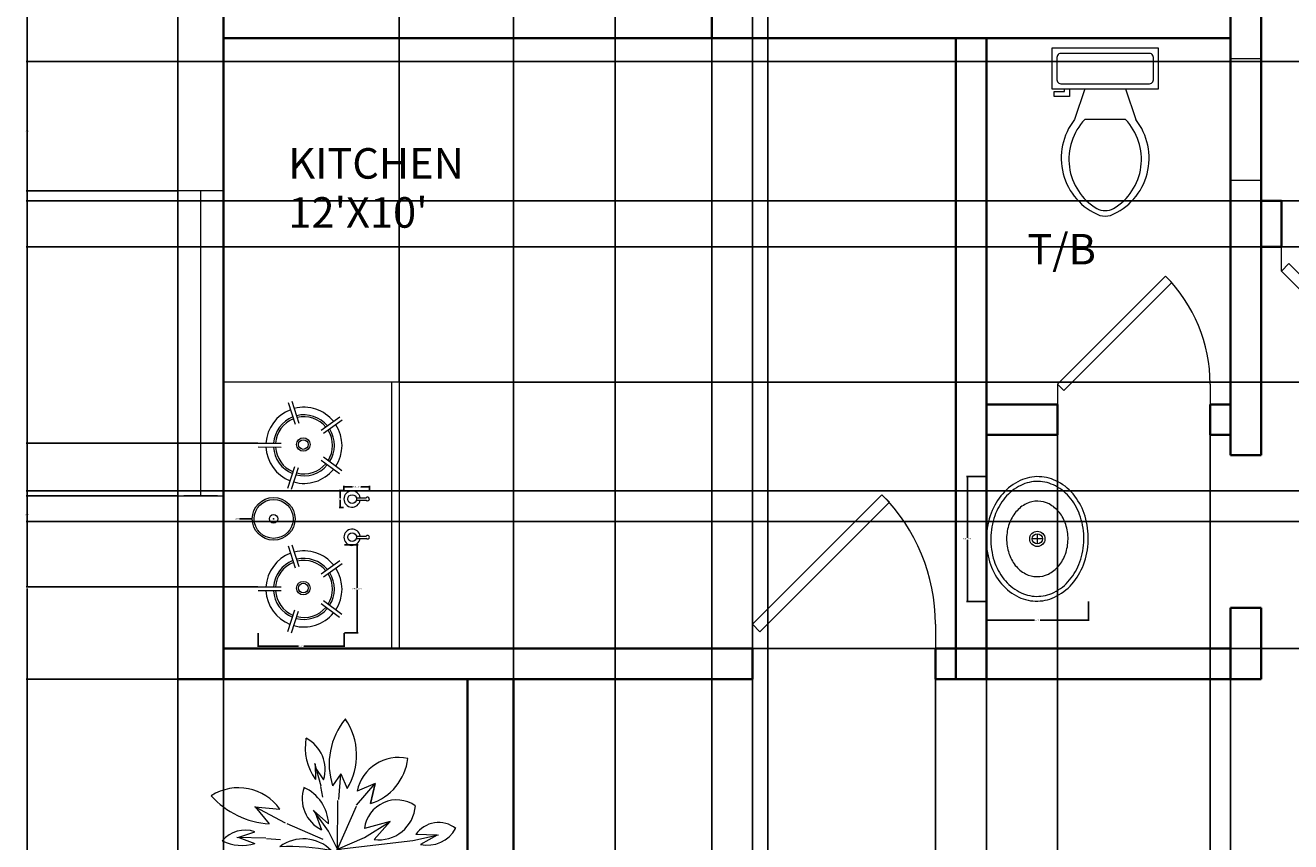
# Model space of a CAD drawing. Units: inches. Extents: x 450 to 1026, y 542 to 1190.
# Tile 8 of 11: x 450 to 698, y 939 to 1099. Entities that reach past the tile are written whole.
import ezdxf

# ---------------------------------------------------------------- set-up
doc = ezdxf.new("R2010")
doc.units = ezdxf.units.IN
doc.header["$MEASUREMENT"] = 0
for name, color, linetype, lineweight in [('A-ANNO-DIMS', 2, 'Continuous', 18), ('A-AREA-IDEN', 7, 'Continuous', 18), ('A-DOOR', 4, 'Continuous', 18), ('A-EQPM', 8, 'Continuous', 18), ('A-FLOR-FIXT', 9, 'Continuous', 18), ('A-GLAZ', 4, 'Continuous', 18), ('A-WALL', 7, 'Continuous', 35), ('C-PROP', 7, 'Continuous', 25), ('L-PLNT', 3, 'Continuous', 13)]:
    doc.layers.add(name, color=color, linetype=linetype, lineweight=lineweight)
doc.styles.get("Standard").update_dxf_attribs({"font": 'arial.ttf'})
doc.dimstyles.get("Standard").update_dxf_attribs({"dimtxt": 0.18, "dimasz": 0.18, "dimexe": 0.18, "dimexo": 0.0625, "dimgap": 0.09, "dimtad": 0, "dimtih": 1, "dimtoh": 1, "dimdec": 4, "dimzin": 0, "dimdsep": 46, "dimtxsty": 'Standard', "dimcen": 0.09, "dimadec": 0, "dimazin": 0, "dimtfac": 1, "dimtdec": 4, "dimtofl": 0, "dimtmove": 0, "dimatfit": 3, "dimfxl": 1, "dimtolj": 1, "dimtzin": 0, "dimarcsym": 0})

# ---------------------------------------------------------------- blocks, each defined once
blk = doc.blocks.new('*U4')
for p, q in [((0, 0), (0, -100)), ((750, 0), (750, -100))]:
    blk.add_line(p, q)
blk.add_lwpolyline([(0, 0), (530.3, 530.3), (561.3, 499.4), (30.9, -30.9)], close=True)
blk.add_arc((0, 0), 750, 0, 45)
blk = doc.blocks.new('*U3')
for p, q in [((0, 100), (0, 0)), ((900, 100), (900, 0)), ((0, 50), (900, 50))]:
    blk.add_line(p, q)
blk = doc.blocks.new('Toilet - top')
for p, q in [((9.5, -6), (9.5, -2)), ((-10, -8.5), (-8, -8.5)), ((-10, -9.5), (-10, -8.5)), ((-7, -9.5), (-10, -9.5)), ((-8, -8.5), (-8, -8)), ((-7, -8), (-7, -9.5)), ((-4, -8), (-6, -14)), ((4, -8), (6, -14)), ((4, -14), (-4, -14))]:
    blk.add_line(p, q)
blk.add_lwpolyline([(10.5, -8), (10.5, 0), (-10.5, 0), (-10.5, -8)], close=True)
for points in [[(-9.5, -2), (-9.5, -6)], [(8.5, -1), (-8.5, -1)], [(-8.5, -7), (8.5, -7)]]:
    blk.add_lwpolyline(points)
for centre, radius, start, end in [((-8.62, -1.88), 0.884, 81.8699, 188.1301), ((8.62, -1.88), 0.884, 351.8699, 98.1301), ((-8.62, -6.12), 0.884, 171.8699, 278.1301), ((8.62, -6.12), 0.884, 261.8699, 8.1301), ((3.52, -21.58), 12.17, 141.4691, 247.9714), ((4.2, -21.82), 11.33, 136.3677, 238.9468), ((-3.52, -21.58), 12.17, 292.0284, 38.5307), ((-4.2, -21.82), 11.33, 301.053, 43.6321), ((0, -27.88), 4, 245.7318, 294.2682), ((0, -29), 4, 254.8605, 285.1395)]:
    blk.add_arc(centre, radius, start, end)
blk = doc.blocks.new('Sink - Oval top')
for p, q in [((-1, 0), (1, 0)), ((0, 1), (0, -1))]:
    blk.add_line(p, q)
for points in [[(-12.23, 0.39, 0.117634), (-11.46, -3.36, 0.104469), (-8.88, -6.8, 0.090016), (-5.08, -9.07, 0.08192), (-0.32, -10.02, 0.08192), (4.49, -9.38, 0.090016), (8.42, -7.36, 0.104469), (11.22, -4.09, 0.117634), (12.23, -0.39, 0.117634), (11.46, 3.36, 0.104469), (8.88, 6.8, 0.090016), (5.08, 9.07, 0.08192), (0.32, 10.02, 0.08192), (-4.49, 9.38, 0.090016), (-8.42, 7.36, 0.104469), (-11.22, 4.09, 0.117634)], [(-11.29, 0.16, 0.118622), (-10.52, -3.25, 0.104678), (-8.07, -6.36, 0.089562), (-4.54, -8.37, 0.081185), (-0.13, -9.15, 0.081185), (4.3, -8.49, 0.089562), (7.89, -6.58, 0.104678), (10.42, -3.55, 0.118622), (11.29, -0.16, 0.118622), (10.52, 3.25, 0.104678), (8.07, 6.36, 0.089562), (4.54, 8.37, 0.081185), (0.13, 9.15, 0.081185), (-4.3, 8.49, 0.089562), (-7.89, 6.58, 0.104678), (-10.42, 3.55, 0.118622)], [(-7.42, 0.08, 0.118283), (-6.91, -2.17, 0.104607), (-5.29, -4.21, 0.089718), (-2.97, -5.53, 0.081436), (-0.07, -6.04, 0.081436), (2.84, -5.59, 0.089718), (5.2, -4.33, 0.104607), (6.86, -2.32, 0.118283), (7.42, -0.08, 0.118283), (6.91, 2.17, 0.104607), (5.29, 4.21, 0.089718), (2.97, 5.53, 0.081436), (0.07, 6.04, 0.081436), (-2.84, 5.59, 0.089718), (-5.2, 4.33, 0.104607), (-6.86, 2.32, 0.118283)]]:
    blk.add_lwpolyline(points, format="xyb", close=True)
for radius in [1.5, 1]:
    blk.add_circle((0, 0), radius)
blk = doc.blocks.new('z_109')
for p, q in [((-93.8, 293.8), (-121.7, 396.4)), ((-120.7, 392.8), (-119, 324)), ((-120.3, 377.4), (-82.1, 322.4)), ((-4.7, 350.4), (-41.8, 295.2)), ((-14.4, 233.6), (-4.7, 350.4)), ((-4.7, 350.4), (24.2, 283.6)), ((-85.3, 244.1), (-94.4, 292.7)), ((65, 208.9), (149.6, 306.7)), ((149.6, 306.7), (68.1, 272.4)), ((129.3, 216), (149.6, 306.7)), ((149.6, 306.7), (129.3, 216)), ((-19.6, 10.5), (-18, 230)), ((-253.8, 128), (-391.6, 201.8)), ((-391.5, 201.8), (-278.3, 190.4)), ((-389.8, 201.6), (-326.7, 125.3)), ((-60.9, 91.7), (-127.6, 186)), ((-126.1, 183.9), (-59.8, 124.6)), ((-120.3, 175.7), (-91.5, 97.7)), ((-19.6, 10.5), (65, 204.6)), ((65, 204.6), (65, 204.6)), ((-83.6, 53.9), (-246.4, 124.8)), ((216.8, 135.4), (101.3, 104.7)), ((101.8, 63.8), (216.8, 135.4)), ((216.8, 135.4), (144.5, 54.6)), ((-342, 60.3), (-471.9, 63)), ((-467.5, 62.9), (-391.6, 89.6)), ((-463.4, 64.3), (-391.5, 36.9)), ((-275.7, 53), (-338.5, 56.9)), ((-19.6, 10.5), (-60.9, 91.7)), ((-19.6, 10.5), (101.8, 63.8)), ((319, 50.5), (433.6, 75.1)), ((428.9, 74.1), (332.5, 76.8)), ((428.1, 74.1), (353.4, 32.3)), ((-19.6, 10.5), (-181.1, -143.2)), ((-19.6, 10.5), (-24.2, -64.6)), ((-19.6, 10.5), (-14.3, 11.4)), ((-14.3, 11.4), (319, 50.5)), ((-14.3, 11.4), (-13.4, 12.7)), ((-13.4, 12.7), (13.4, -12.7)), ((-177.8, -41.4), (-312.5, -91.6)), ((-308.1, -89.9), (-254.4, -32.6)), ((-86.1, -7.9), (-177.8, -41.4)), ((15.9, -43.2), (88.2, -126.5)), ((122.5, -7.9), (193.1, -11)), ((176.2, -10.2), (284.5, -54.4)), ((283.1, -53.8), (196.2, -42.2)), ((272.8, -52.5), (222, -4.2)), ((-305.8, -89.1), (-217, -88.2)), ((-25.6, -113), (-45, -65.8)), ((-24.2, -64.6), (-28.2, -121)), ((-27.9, -117.3), (-2.3, -69.4)), ((-186.9, -142.9), (-344.9, -240)), ((-342.2, -238.3), (-268.6, -151.1)), ((141.1, -208), (83.6, -170.3)), ((87.3, -129.3), (139.6, -204.2)), ((140.4, -205.5), (123.1, -139.2)), ((-328.5, -229.9), (-213.2, -194.7)), ((-88.6, -191.8), (-150.4, -266.6)), ((-149.9, -266), (-130.8, -198.8)), ((3.5, -191.8), (15.9, -238.1)), ((-150.6, -266.9), (-80.7, -228.2)), ((33.8, -320.1), (-6.3, -268.4)), ((15.9, -238.1), (35.2, -326.4)), ((35.2, -326.5), (45.1, -249.3))]:
    blk.add_line(p, q)
for centre, radius, start, end in [((262.2, 393.4), 319.4, 140.563, 197.8988), ((-221.5, 433.3), 287.6, 328.6458, 34.5329), ((84.2, 468), 249.1, 170.3029, 215.3262), ((-234.9, 368.4), 159.6, 343.2534, 62.5239), ((255.6, 231.5), 191.8, 77.7318, 167.6805), ((55.5, 446.9), 242.5, 287.7269, 353.3689), ((-464.4, 59.2), 227.7, 35.1725, 122.5976), ((-20.9, 238.7), 157.6, 161.4501, 243.415), ((-251.5, 114.8), 192, 2.9136, 65.0019), ((-304.3, 504.2), 379.6, 221.8384, 266.6027), ((246.7, 85.9), 146.6, 55.2824, 172.6291), ((166.6, 217.1), 164, 262.2896, 356.2544), ((434.4, 8.1), 122.9, 51.1111, 145.9654), ((-434.4, -39.4), 135.9, 71.6414, 139.5892), ((-172.9, -117.6), 175.2, 44.3837, 127.1057), ((384.1, 175.1), 146, 257.8549, 330.7421), ((-450, 225.2), 197.1, 243.5199, 287.2599), ((-243.2, -1062.9), 1085.6, 79.6239, 91.8656), ((-246.3, -222.4), 190, 92.4489, 147.0817), ((52.6, -110.1), 105, 354.7987, 111.9005), ((1.6, -181.5), 167.4, 21.6922, 85.2277), ((324.6, 60.3), 164.3, 218.6232, 288.4099), ((240.6, -148.9), 145.9, 21.4559, 97.3107), ((-336.9, 52.1), 184.6, 248.0932, 310.529), ((-31.3, -123), 58.9, 103.4106, 268.148), ((-25.7, -123.5), 58.9, 262.5922, 66.6581), ((-198.2, -444.5), 301.7, 103.499, 156.8265), ((196.5, -160), 113.4, 185.1842, 278.9266), ((66, -275.9), 148.2, 1.4924, 67.3596), ((-454.6, -39.5), 287, 265.8156, 327.2626), ((-93.8, -301), 108.7, 109.8936, 199.3062), ((-186.1, -231.9), 105.5, 264.4232, 2.0221), ((80, -308.4), 95.1, 155.1092, 275.9038), ((-27.8, -353.9), 127.5, 337.3115, 55.0978)]:
    blk.add_arc(centre, radius, start, end)
blk = doc.blocks.new('COOKTOP-BURNER')
for p, q in [((5.9, 17.07), (7.26, 12.79)), ((6.61, 17.3), (7.98, 13.01)), ((16.05, 14.17), (12.39, 11.54)), ((16.49, 13.56), (12.83, 10.94)), ((0, 9.07), (4.5, 9.04)), ((0, 8.32), (4.5, 8.29)), ((15.98, 3.01), (12.36, 5.68)), ((16.42, 3.61), (12.8, 6.28)), ((5.79, 0.24), (7.21, 4.5)), ((6.5, 0), (7.92, 4.27))]:
    blk.add_line(p, q)
for radius in [1.33, 0.951]:
    blk.add_circle((8.85, 8.79), radius)
for radius, start, end in [(7.48, 110.4975, 176.7655), (7.48, 38.4975, 104.7655), (5.99, 111.454, 175.8089), (5.61, 111.454, 175.8089), (5.99, 39.454, 103.8089), (5.61, 39.454, 103.8089), (7.48, 326.4975, 32.7655), (5.61, 327.454, 31.8089), (5.99, 327.454, 31.8089), (7.48, 182.4975, 248.7655), (5.99, 183.454, 247.8089), (5.61, 183.454, 247.8089), (5.61, 255.454, 319.8089), (7.48, 254.4975, 320.7655), (5.99, 255.454, 319.8089)]:
    blk.add_arc((8.98, 8.63), radius, start, end)
blk = doc.blocks.new('COOKTOP-CONTROL')
for p, q in [((2.42, 1.83), (4.35, 1.83)), ((2.43, 1.38), (4.37, 1.38))]:
    blk.add_line(p, q)
blk.add_circle((1.6, 1.6), 0.854)
for centre, radius, start, end in [((1.6, 1.6), 1.6, 8.1625, 352.0201), ((4.64, 1.62), 0.361, 220.6048, 143.5533)]:
    blk.add_arc(centre, radius, start, end)
blk = doc.blocks.new('*D33')
at = {"layer": 'A-ANNO-DIMS', "color": 0, "lineweight": -2, "transparency": 16777216}
for p, q in [((638.54, 1010.78), (634.74, 1010.78)), ((634.92, 1010.6), (634.92, 998.69)), ((634.92, 986.41), (634.92, 998.32)), ((638.54, 986.23), (634.74, 986.23))]:
    blk.add_line(p, q, dxfattribs=at)
at = {"layer": 'A-ANNO-DIMS', "color": 0, "transparency": 16777216}
for points in [[(634.89, 1010.6), (634.95, 1010.6), (634.92, 1010.78)], [(634.89, 986.41), (634.95, 986.41), (634.92, 986.23)]]:
    blk.add_solid(points, dxfattribs=at)
at = {"layer": 'Defpoints', "color": 0, "transparency": 16777216}
for p in [(638.6, 1010.78), (634.92, 986.23), (638.6, 986.23)]:
    blk.add_point(p, dxfattribs=at)
at = {"layer": 'A-ANNO-DIMS', "color": 0, "transparency": 16777216, "insert": (634.92, 998.51), "char_height": 0.18, "attachment_point": 5}
blk.add_mtext('\\A1;BASIN 25 TYP.', dxfattribs=at)
blk = doc.blocks.new('*D34')
at = {"layer": 'A-ANNO-DIMS', "color": 0, "lineweight": -2, "transparency": 16777216}
for p, q in [((638.6, 986.17), (638.6, 982.37)), ((658.74, 986.17), (658.74, 982.37)), ((638.78, 982.55), (648.14, 982.55)), ((658.56, 982.55), (649.2, 982.55))]:
    blk.add_line(p, q, dxfattribs=at)
at = {"layer": 'A-ANNO-DIMS', "color": 0, "transparency": 16777216}
for points in [[(638.78, 982.58), (638.78, 982.52), (638.6, 982.55)], [(658.56, 982.58), (658.56, 982.52), (658.74, 982.55)]]:
    blk.add_solid(points, dxfattribs=at)
at = {"layer": 'Defpoints', "color": 0, "transparency": 16777216}
for p in [(638.6, 986.23), (658.74, 986.23), (658.74, 982.55)]:
    blk.add_point(p, dxfattribs=at)
at = {"layer": 'A-ANNO-DIMS', "color": 0, "transparency": 16777216, "insert": (648.67, 982.55), "char_height": 0.18, "attachment_point": 5}
blk.add_mtext('\\A1;20 TYP.', dxfattribs=at)
blk = doc.blocks.new('*D39')
at = {"layer": 'A-ANNO-DIMS', "color": 0, "lineweight": -2, "transparency": 16777216}
for p, q in [((512.43, 997.34), (515.14, 997.34)), ((514.96, 997.16), (514.96, 988.87)), ((514.96, 980.22), (514.96, 988.51)), ((512.43, 980.04), (515.14, 980.04))]:
    blk.add_line(p, q, dxfattribs=at)
at = {"layer": 'A-ANNO-DIMS', "color": 0, "transparency": 16777216}
for points in [[(514.93, 997.16), (514.99, 997.16), (514.96, 997.34)], [(514.93, 980.22), (514.99, 980.22), (514.96, 980.04)]]:
    blk.add_solid(points, dxfattribs=at)
at = {"layer": 'Defpoints', "color": 0, "transparency": 16777216}
for p in [(512.36, 997.34), (514.96, 997.34), (512.36, 980.04)]:
    blk.add_point(p, dxfattribs=at)
at = {"layer": 'A-ANNO-DIMS', "color": 0, "transparency": 16777216, "insert": (514.96, 988.69), "char_height": 0.18, "attachment_point": 5}
blk.add_mtext('\\A1;BURNER 17 TYP.', dxfattribs=at)
blk = doc.blocks.new('*D40')
at = {"layer": 'A-ANNO-DIMS', "color": 0, "lineweight": -2, "transparency": 16777216}
for p, q in [((495.49, 979.98), (495.49, 977.27)), ((512.36, 979.98), (512.36, 977.27)), ((495.67, 977.45), (503.41, 977.45)), ((512.18, 977.45), (504.45, 977.45))]:
    blk.add_line(p, q, dxfattribs=at)
at = {"layer": 'A-ANNO-DIMS', "color": 0, "transparency": 16777216}
for points in [[(495.67, 977.48), (495.67, 977.42), (495.49, 977.45)], [(512.18, 977.48), (512.18, 977.42), (512.36, 977.45)]]:
    blk.add_solid(points, dxfattribs=at)
at = {"layer": 'Defpoints', "color": 0, "transparency": 16777216}
for p in [(495.49, 980.04), (512.36, 980.04), (512.36, 977.45)]:
    blk.add_point(p, dxfattribs=at)
at = {"layer": 'A-ANNO-DIMS', "color": 0, "transparency": 16777216, "insert": (503.93, 977.45), "char_height": 0.18, "attachment_point": 5}
blk.add_mtext('\\A1;17 TYP.', dxfattribs=at)
blk = doc.blocks.new('*D41')
at = {"layer": 'A-ANNO-DIMS', "color": 0, "lineweight": -2, "transparency": 16777216}
for p, q in [((512.32, 1008.07), (512.32, 1008.94)), ((512.5, 1008.76), (513.98, 1008.76)), ((517.15, 1008.76), (515.67, 1008.76)), ((517.33, 1008.07), (517.33, 1008.94))]:
    blk.add_line(p, q, dxfattribs=at)
at = {"layer": 'A-ANNO-DIMS', "color": 0, "transparency": 16777216}
for points in [[(512.5, 1008.79), (512.5, 1008.73), (512.32, 1008.76)], [(517.15, 1008.79), (517.15, 1008.73), (517.33, 1008.76)]]:
    blk.add_solid(points, dxfattribs=at)
at = {"layer": 'Defpoints', "color": 0, "transparency": 16777216}
for p in [(512.32, 1008.01), (517.33, 1008.76), (517.33, 1008.01)]:
    blk.add_point(p, dxfattribs=at)
at = {"layer": 'A-ANNO-DIMS', "color": 0, "transparency": 16777216, "insert": (514.83, 1008.76), "char_height": 0.18, "attachment_point": 5}
blk.add_mtext('\\A1;KNOB 5 TYP.', dxfattribs=at)
blk = doc.blocks.new('*D42')
at = {"layer": 'A-ANNO-DIMS', "color": 0, "lineweight": -2, "transparency": 16777216}
for p, q in [((512.26, 1008.01), (511.39, 1008.01)), ((511.57, 1007.83), (511.57, 1006.53)), ((511.57, 1004.87), (511.57, 1006.17)), ((512.26, 1004.69), (511.39, 1004.69))]:
    blk.add_line(p, q, dxfattribs=at)
at = {"layer": 'A-ANNO-DIMS', "color": 0, "transparency": 16777216}
for points in [[(511.54, 1007.83), (511.6, 1007.83), (511.57, 1008.01)], [(511.54, 1004.87), (511.6, 1004.87), (511.57, 1004.69)]]:
    blk.add_solid(points, dxfattribs=at)
at = {"layer": 'Defpoints', "color": 0, "transparency": 16777216}
for p in [(511.57, 1008.01), (512.32, 1008.01), (512.32, 1004.69)]:
    blk.add_point(p, dxfattribs=at)
at = {"layer": 'A-ANNO-DIMS', "color": 0, "transparency": 16777216, "insert": (511.57, 1006.35), "char_height": 0.18, "attachment_point": 5}
blk.add_mtext('\\A1;3 TYP.', dxfattribs=at)
blk = doc.blocks.new('*D47')
at = {"layer": 'A-ANNO-DIMS', "color": 0, "lineweight": -2, "transparency": 16777216}
for p, q in [((479.65, 1160.01), (479.65, 1189.72)), ((479.83, 1189.54), (719.36, 1189.54)), ((959.47, 1189.54), (719.94, 1189.54)), ((959.65, 1065.01), (959.65, 1189.72))]:
    blk.add_line(p, q, dxfattribs=at)
at = {"layer": 'A-ANNO-DIMS', "color": 0, "transparency": 16777216}
for points in [[(479.83, 1189.57), (479.83, 1189.51), (479.65, 1189.54)], [(959.47, 1189.57), (959.47, 1189.51), (959.65, 1189.54)]]:
    blk.add_solid(points, dxfattribs=at)
at = {"layer": 'Defpoints', "color": 0, "transparency": 16777216}
for p in [(959.65, 1189.54), (479.65, 1159.94), (959.65, 1064.94)]:
    blk.add_point(p, dxfattribs=at)
at = {"layer": 'A-ANNO-DIMS', "color": 0, "transparency": 16777216, "insert": (719.65, 1189.54), "char_height": 0.18, "attachment_point": 5}
blk.add_mtext('\\A1;480', dxfattribs=at)
blk = doc.blocks.new('*D49')
at = {"layer": 'A-ANNO-DIMS', "color": 0, "lineweight": -2, "transparency": 16777216}
for p, q in [((479.59, 1159.94), (449.87, 1159.94)), ((450.05, 1159.76), (450.05, 1113.62)), ((450.05, 1067.12), (450.05, 1113.26)), ((479.59, 1066.94), (449.87, 1066.94))]:
    blk.add_line(p, q, dxfattribs=at)
at = {"layer": 'A-ANNO-DIMS', "color": 0, "transparency": 16777216}
for points in [[(450.02, 1159.76), (450.08, 1159.76), (450.05, 1159.94)], [(450.02, 1067.12), (450.08, 1067.12), (450.05, 1066.94)]]:
    blk.add_solid(points, dxfattribs=at)
at = {"layer": 'Defpoints', "color": 0, "transparency": 16777216}
for p in [(479.65, 1159.94), (450.05, 1066.94), (479.65, 1066.94)]:
    blk.add_point(p, dxfattribs=at)
at = {"layer": 'A-ANNO-DIMS', "color": 0, "transparency": 16777216, "insert": (450.05, 1113.44), "char_height": 0.18, "attachment_point": 5}
blk.add_mtext('\\A1;93', dxfattribs=at)
blk = doc.blocks.new('*D50')
at = {"layer": 'A-ANNO-DIMS', "color": 0, "lineweight": -2, "transparency": 16777216}
for p, q in [((479.59, 1066.94), (449.87, 1066.94)), ((450.05, 1066.76), (450.05, 1037.12)), ((450.05, 1007.12), (450.05, 1036.76)), ((479.59, 1006.94), (449.87, 1006.94))]:
    blk.add_line(p, q, dxfattribs=at)
at = {"layer": 'A-ANNO-DIMS', "color": 0, "transparency": 16777216}
for points in [[(450.02, 1066.76), (450.08, 1066.76), (450.05, 1066.94)], [(450.02, 1007.12), (450.08, 1007.12), (450.05, 1006.94)]]:
    blk.add_solid(points, dxfattribs=at)
at = {"layer": 'Defpoints', "color": 0, "transparency": 16777216}
for p in [(479.65, 1066.94), (450.05, 1006.94), (479.65, 1006.94)]:
    blk.add_point(p, dxfattribs=at)
at = {"layer": 'A-ANNO-DIMS', "color": 0, "transparency": 16777216, "insert": (450.05, 1036.94), "char_height": 0.18, "attachment_point": 5}
blk.add_mtext('\\A1;60', dxfattribs=at)
blk = doc.blocks.new('*D51')
at = {"layer": 'A-ANNO-DIMS', "color": 0, "lineweight": -2, "transparency": 16777216}
for p, q in [((479.59, 1006.94), (449.87, 1006.94)), ((450.05, 1006.76), (450.05, 989.12)), ((450.05, 971.12), (450.05, 988.76)), ((479.59, 970.94), (449.87, 970.94))]:
    blk.add_line(p, q, dxfattribs=at)
at = {"layer": 'A-ANNO-DIMS', "color": 0, "transparency": 16777216}
for points in [[(450.02, 1006.76), (450.08, 1006.76), (450.05, 1006.94)], [(450.02, 971.12), (450.08, 971.12), (450.05, 970.94)]]:
    blk.add_solid(points, dxfattribs=at)
at = {"layer": 'Defpoints', "color": 0, "transparency": 16777216}
for p in [(479.65, 1006.94), (450.05, 970.94), (479.65, 970.94)]:
    blk.add_point(p, dxfattribs=at)
at = {"layer": 'A-ANNO-DIMS', "color": 0, "transparency": 16777216, "insert": (450.05, 988.94), "char_height": 0.18, "attachment_point": 5}
blk.add_mtext('\\A1;36', dxfattribs=at)
blk = doc.blocks.new('*D52')
at = {"layer": 'A-ANNO-DIMS', "color": 0, "lineweight": -2, "transparency": 16777216}
for p, q in [((479.59, 970.94), (449.87, 970.94)), ((450.05, 970.76), (450.05, 894.62)), ((450.05, 818.12), (450.05, 894.26)), ((479.59, 817.94), (449.87, 817.94))]:
    blk.add_line(p, q, dxfattribs=at)
at = {"layer": 'A-ANNO-DIMS', "color": 0, "transparency": 16777216}
for points in [[(450.02, 970.76), (450.08, 970.76), (450.05, 970.94)], [(450.02, 818.12), (450.08, 818.12), (450.05, 817.94)]]:
    blk.add_solid(points, dxfattribs=at)
at = {"layer": 'Defpoints', "color": 0, "transparency": 16777216}
for p in [(479.65, 970.94), (450.05, 817.94), (479.65, 817.94)]:
    blk.add_point(p, dxfattribs=at)
at = {"layer": 'A-ANNO-DIMS', "color": 0, "transparency": 16777216, "insert": (450.05, 894.44), "char_height": 0.18, "attachment_point": 5}
blk.add_mtext('\\A1;153', dxfattribs=at)
blk = doc.blocks.new('*D55')
at = {"layer": 'A-ANNO-DIMS', "color": 0, "lineweight": -2, "transparency": 16777216}
for p, q in [((995.59, 1159.94), (449.87, 1159.94)), ((450.05, 1159.76), (450.05, 1112.62)), ((450.05, 1065.12), (450.05, 1112.26)), ((959.59, 1064.94), (449.87, 1064.94))]:
    blk.add_line(p, q, dxfattribs=at)
at = {"layer": 'A-ANNO-DIMS', "color": 0, "transparency": 16777216}
for points in [[(450.02, 1159.76), (450.08, 1159.76), (450.05, 1159.94)], [(450.02, 1065.12), (450.08, 1065.12), (450.05, 1064.94)]]:
    blk.add_solid(points, dxfattribs=at)
at = {"layer": 'Defpoints', "color": 0, "transparency": 16777216}
for p in [(995.65, 1159.94), (450.05, 1064.94), (959.65, 1064.94)]:
    blk.add_point(p, dxfattribs=at)
at = {"layer": 'A-ANNO-DIMS', "color": 0, "transparency": 16777216, "insert": (450.05, 1112.44), "char_height": 0.18, "attachment_point": 5}
blk.add_mtext('\\A1;95', dxfattribs=at)
blk = doc.blocks.new('*D56')
at = {"layer": 'A-ANNO-DIMS', "color": 0, "lineweight": -2, "transparency": 16777216}
for p, q in [((488.65, 1150.88), (488.65, 542.16)), ((584.65, 1150.88), (584.65, 542.16)), ((488.83, 542.34), (536.43, 542.34)), ((584.47, 542.34), (536.87, 542.34))]:
    blk.add_line(p, q, dxfattribs=at)
at = {"layer": 'A-ANNO-DIMS', "color": 0, "transparency": 16777216}
for points in [[(488.83, 542.37), (488.83, 542.31), (488.65, 542.34)], [(584.47, 542.37), (584.47, 542.31), (584.65, 542.34)]]:
    blk.add_solid(points, dxfattribs=at)
at = {"layer": 'Defpoints', "color": 0, "transparency": 16777216}
for p in [(488.65, 1150.94), (584.65, 1150.94), (584.65, 542.34)]:
    blk.add_point(p, dxfattribs=at)
at = {"layer": 'A-ANNO-DIMS', "color": 0, "transparency": 16777216, "insert": (536.65, 542.34), "char_height": 0.18, "attachment_point": 5}
blk.add_mtext('\\A1;96', dxfattribs=at)
blk = doc.blocks.new('*D57')
at = {"layer": 'A-ANNO-DIMS', "color": 0, "lineweight": -2, "transparency": 16777216}
for p, q in [((638.65, 970.88), (638.65, 542.16)), ((686.65, 970.88), (686.65, 542.16)), ((638.83, 542.34), (662.43, 542.34)), ((686.47, 542.34), (662.87, 542.34))]:
    blk.add_line(p, q, dxfattribs=at)
at = {"layer": 'A-ANNO-DIMS', "color": 0, "transparency": 16777216}
for points in [[(638.83, 542.37), (638.83, 542.31), (638.65, 542.34)], [(686.47, 542.37), (686.47, 542.31), (686.65, 542.34)]]:
    blk.add_solid(points, dxfattribs=at)
at = {"layer": 'Defpoints', "color": 0, "transparency": 16777216}
for p in [(638.65, 970.94), (686.65, 970.94), (686.65, 542.34)]:
    blk.add_point(p, dxfattribs=at)
at = {"layer": 'A-ANNO-DIMS', "color": 0, "transparency": 16777216, "insert": (662.65, 542.34), "char_height": 0.18, "attachment_point": 5}
blk.add_mtext('\\A1;48', dxfattribs=at)
blk = doc.blocks.new('*D58')
at = {"layer": 'A-ANNO-DIMS', "color": 0, "lineweight": -2, "transparency": 16777216}
for p, q in [((545.65, 971.01), (545.65, 1189.72)), ((545.83, 1189.54), (568.93, 1189.54)), ((592.47, 1189.54), (569.37, 1189.54)), ((592.65, 977.01), (592.65, 1189.72))]:
    blk.add_line(p, q, dxfattribs=at)
at = {"layer": 'A-ANNO-DIMS', "color": 0, "transparency": 16777216}
for points in [[(545.83, 1189.57), (545.83, 1189.51), (545.65, 1189.54)], [(592.47, 1189.57), (592.47, 1189.51), (592.65, 1189.54)]]:
    blk.add_solid(points, dxfattribs=at)
at = {"layer": 'Defpoints', "color": 0, "transparency": 16777216}
for p in [(592.65, 1189.54), (592.65, 976.94), (545.65, 970.94)]:
    blk.add_point(p, dxfattribs=at)
at = {"layer": 'A-ANNO-DIMS', "color": 0, "transparency": 16777216, "insert": (569.15, 1189.54), "char_height": 0.18, "attachment_point": 5}
blk.add_mtext('\\A1;47', dxfattribs=at)
blk = doc.blocks.new('*D62')
at = {"layer": 'A-ANNO-DIMS', "color": 0, "lineweight": -2, "transparency": 16777216}
for p, q in [((771.36, 1055.94), (449.87, 1055.94)), ((450.05, 1055.76), (450.05, 1032.12)), ((450.05, 1008.12), (450.05, 1031.76)), ((771.36, 1007.94), (449.87, 1007.94))]:
    blk.add_line(p, q, dxfattribs=at)
at = {"layer": 'A-ANNO-DIMS', "color": 0, "transparency": 16777216}
for points in [[(450.02, 1055.76), (450.08, 1055.76), (450.05, 1055.94)], [(450.02, 1008.12), (450.08, 1008.12), (450.05, 1007.94)]]:
    blk.add_solid(points, dxfattribs=at)
at = {"layer": 'Defpoints', "color": 0, "transparency": 16777216}
for p in [(771.42, 1055.94), (450.05, 1007.94), (771.42, 1007.94)]:
    blk.add_point(p, dxfattribs=at)
at = {"layer": 'A-ANNO-DIMS', "color": 0, "transparency": 16777216, "insert": (450.05, 1031.94), "char_height": 0.18, "attachment_point": 5}
blk.add_mtext('\\A1;48', dxfattribs=at)
blk = doc.blocks.new('*D63')
at = {"layer": 'A-ANNO-DIMS', "color": 0, "lineweight": -2, "transparency": 16777216}
for p, q in [((771.36, 1092.35), (449.87, 1092.35)), ((450.05, 1092.17), (450.05, 1078.83)), ((450.05, 1065.12), (450.05, 1078.47)), ((771.36, 1064.94), (449.87, 1064.94))]:
    blk.add_line(p, q, dxfattribs=at)
at = {"layer": 'A-ANNO-DIMS', "color": 0, "transparency": 16777216}
for points in [[(450.02, 1092.17), (450.08, 1092.17), (450.05, 1092.35)], [(450.02, 1065.12), (450.08, 1065.12), (450.05, 1064.94)]]:
    blk.add_solid(points, dxfattribs=at)
at = {"layer": 'Defpoints', "color": 0, "transparency": 16777216}
for p in [(771.42, 1092.35), (450.05, 1064.94), (771.42, 1064.94)]:
    blk.add_point(p, dxfattribs=at)
at = {"layer": 'A-ANNO-DIMS', "color": 0, "transparency": 16777216, "insert": (450.05, 1078.65), "char_height": 0.18, "attachment_point": 5}
blk.add_mtext('\\A1;27.41', dxfattribs=at)
blk = doc.blocks.new('*D65')
at = {"layer": 'A-ANNO-DIMS', "color": 0, "lineweight": -2, "transparency": 16777216}
for p, q in [((592.65, 970.88), (592.65, 542.16)), ((628.65, 970.88), (628.65, 542.16)), ((592.83, 542.34), (610.43, 542.34)), ((628.47, 542.34), (610.87, 542.34))]:
    blk.add_line(p, q, dxfattribs=at)
at = {"layer": 'A-ANNO-DIMS', "color": 0, "transparency": 16777216}
for points in [[(592.83, 542.37), (592.83, 542.31), (592.65, 542.34)], [(628.47, 542.37), (628.47, 542.31), (628.65, 542.34)]]:
    blk.add_solid(points, dxfattribs=at)
at = {"layer": 'Defpoints', "color": 0, "transparency": 16777216}
for p in [(592.65, 970.94), (628.65, 970.94), (628.65, 542.34)]:
    blk.add_point(p, dxfattribs=at)
at = {"layer": 'A-ANNO-DIMS', "color": 0, "transparency": 16777216, "insert": (610.65, 542.34), "char_height": 0.18, "attachment_point": 5}
blk.add_mtext('\\A1;36', dxfattribs=at)
blk = doc.blocks.new('*D66')
at = {"layer": 'A-ANNO-DIMS', "color": 0, "lineweight": -2, "transparency": 16777216}
for p, q in [((652.65, 1018.88), (652.65, 542.16)), ((682.65, 1018.88), (682.65, 542.16)), ((652.83, 542.34), (667.43, 542.34)), ((682.47, 542.34), (667.87, 542.34))]:
    blk.add_line(p, q, dxfattribs=at)
at = {"layer": 'A-ANNO-DIMS', "color": 0, "transparency": 16777216}
for points in [[(652.83, 542.37), (652.83, 542.31), (652.65, 542.34)], [(682.47, 542.37), (682.47, 542.31), (682.65, 542.34)]]:
    blk.add_solid(points, dxfattribs=at)
at = {"layer": 'Defpoints', "color": 0, "transparency": 16777216}
for p in [(652.65, 1018.94), (682.65, 1018.94), (682.65, 542.34)]:
    blk.add_point(p, dxfattribs=at)
at = {"layer": 'A-ANNO-DIMS', "color": 0, "transparency": 16777216, "insert": (667.65, 542.34), "char_height": 0.18, "attachment_point": 5}
blk.add_mtext('\\A1;30', dxfattribs=at)
blk = doc.blocks.new('*D67')
at = {"layer": 'A-ANNO-DIMS', "color": 0, "lineweight": -2, "transparency": 16777216}
for p, q in [((488.65, 1029.39), (488.65, 1189.72)), ((488.83, 1189.54), (505.54, 1189.54)), ((523.04, 1189.54), (506.33, 1189.54)), ((523.22, 1029.39), (523.22, 1189.72))]:
    blk.add_line(p, q, dxfattribs=at)
at = {"layer": 'A-ANNO-DIMS', "color": 0, "transparency": 16777216}
for points in [[(488.83, 1189.57), (488.83, 1189.51), (488.65, 1189.54)], [(523.04, 1189.57), (523.04, 1189.51), (523.22, 1189.54)]]:
    blk.add_solid(points, dxfattribs=at)
at = {"layer": 'Defpoints', "color": 0, "transparency": 16777216}
for p in [(523.22, 1189.54), (488.65, 1029.33), (523.22, 1029.33)]:
    blk.add_point(p, dxfattribs=at)
at = {"layer": 'A-ANNO-DIMS', "color": 0, "transparency": 16777216, "insert": (505.94, 1189.54), "char_height": 0.18, "attachment_point": 5}
blk.add_mtext('\\A1;34.57', dxfattribs=at)
blk = doc.blocks.new('*D68')
at = {"layer": 'A-ANNO-DIMS', "color": 0, "lineweight": -2, "transparency": 16777216}
for p, q in [((523.29, 1029.33), (1025.43, 1029.33)), ((1025.25, 1029.15), (1025.25, 1003.32)), ((1025.25, 977.12), (1025.25, 1002.96)), ((523.29, 976.94), (1025.43, 976.94))]:
    blk.add_line(p, q, dxfattribs=at)
at = {"layer": 'A-ANNO-DIMS', "color": 0, "transparency": 16777216}
for points in [[(1025.22, 1029.15), (1025.28, 1029.15), (1025.25, 1029.33)], [(1025.22, 977.12), (1025.28, 977.12), (1025.25, 976.94)]]:
    blk.add_solid(points, dxfattribs=at)
at = {"layer": 'Defpoints', "color": 0, "transparency": 16777216}
for p in [(523.22, 1029.33), (1025.25, 1029.33), (523.22, 976.94)]:
    blk.add_point(p, dxfattribs=at)
at = {"layer": 'A-ANNO-DIMS', "color": 0, "transparency": 16777216, "insert": (1025.25, 1003.14), "char_height": 0.18, "attachment_point": 5}
blk.add_mtext('\\A1;52.39', dxfattribs=at)
blk = doc.blocks.new('*D69')
at = {"layer": 'A-ANNO-DIMS', "color": 0, "lineweight": -2, "transparency": 16777216}
for p, q in [((495.43, 1017.33), (449.87, 1017.33)), ((450.05, 1017.15), (450.05, 1003.4)), ((450.05, 989.29), (450.05, 1003.04)), ((495.43, 989.11), (449.87, 989.11))]:
    blk.add_line(p, q, dxfattribs=at)
at = {"layer": 'A-ANNO-DIMS', "color": 0, "transparency": 16777216}
for points in [[(450.02, 1017.15), (450.08, 1017.15), (450.05, 1017.33)], [(450.02, 989.29), (450.08, 989.29), (450.05, 989.11)]]:
    blk.add_solid(points, dxfattribs=at)
at = {"layer": 'Defpoints', "color": 0, "transparency": 16777216}
for p in [(495.49, 1017.33), (450.05, 989.11), (495.49, 989.11)]:
    blk.add_point(p, dxfattribs=at)
at = {"layer": 'A-ANNO-DIMS', "color": 0, "transparency": 16777216, "insert": (450.05, 1003.22), "char_height": 0.18, "attachment_point": 5}
blk.add_mtext('\\A1;28.224', dxfattribs=at)
blk = doc.blocks.new('*D70')
at = {"layer": 'A-ANNO-DIMS', "color": 0, "lineweight": -2, "transparency": 16777216}
for p, q in [((565.65, 713.01), (565.65, 1189.72)), ((565.83, 1189.54), (580.43, 1189.54)), ((595.47, 1189.54), (580.87, 1189.54)), ((595.65, 713.01), (595.65, 1189.72))]:
    blk.add_line(p, q, dxfattribs=at)
at = {"layer": 'A-ANNO-DIMS', "color": 0, "transparency": 16777216}
for points in [[(565.83, 1189.57), (565.83, 1189.51), (565.65, 1189.54)], [(595.47, 1189.57), (595.47, 1189.51), (595.65, 1189.54)]]:
    blk.add_solid(points, dxfattribs=at)
at = {"layer": 'Defpoints', "color": 0, "transparency": 16777216}
for p in [(595.65, 1189.54), (565.65, 712.94), (595.65, 712.94)]:
    blk.add_point(p, dxfattribs=at)
at = {"layer": 'A-ANNO-DIMS', "color": 0, "transparency": 16777216, "insert": (580.65, 1189.54), "char_height": 0.18, "attachment_point": 5}
blk.add_mtext('\\A1;30', dxfattribs=at)
blk = doc.blocks.new('*D74')
at = {"layer": 'A-ANNO-DIMS', "color": 0, "lineweight": -2, "transparency": 16777216}
for p, q in [((959.59, 1055.94), (449.87, 1055.94)), ((450.05, 1055.76), (450.05, 1029.12)), ((450.05, 1002.12), (450.05, 1028.76)), ((950.59, 1001.94), (449.87, 1001.94))]:
    blk.add_line(p, q, dxfattribs=at)
at = {"layer": 'A-ANNO-DIMS', "color": 0, "transparency": 16777216}
for points in [[(450.02, 1055.76), (450.08, 1055.76), (450.05, 1055.94)], [(450.02, 1002.12), (450.08, 1002.12), (450.05, 1001.94)]]:
    blk.add_solid(points, dxfattribs=at)
at = {"layer": 'Defpoints', "color": 0, "transparency": 16777216}
for p in [(450.05, 1055.94), (959.65, 1055.94), (950.65, 1001.94)]:
    blk.add_point(p, dxfattribs=at)
at = {"layer": 'A-ANNO-DIMS', "color": 0, "transparency": 16777216, "insert": (450.05, 1028.94), "char_height": 0.18, "attachment_point": 5}
blk.add_mtext('\\A1;54', dxfattribs=at)
blk = doc.blocks.new('*D77')
at = {"layer": 'A-ANNO-DIMS', "color": 0, "lineweight": -2, "transparency": 16777216}
for p, q in [((491.77, 1002.45), (494.12, 1002.45)), ((498.41, 1002.45), (498.59, 1002.45)), ((498.5, 1002.36), (498.5, 1002.54))]:
    blk.add_line(p, q, dxfattribs=at)
at = {"layer": 'A-ANNO-DIMS', "color": 0, "transparency": 16777216}
blk.add_solid([(494.12, 1002.48), (494.12, 1002.42), (494.3, 1002.45)], dxfattribs=at)
at = {"layer": 'Defpoints', "color": 0, "transparency": 16777216}
for p in [(494.3, 1002.45), (502.71, 1002.45)]:
    blk.add_point(p, dxfattribs=at)
at = {"layer": 'A-ANNO-DIMS', "color": 0, "transparency": 16777216, "insert": (491.28, 1002.45), "char_height": 0.18, "attachment_point": 5}
blk.add_mtext('\\A1;∅8.412', dxfattribs=at)

msp = doc.modelspace()

# ---------------------------------------------------------------- linework, layer by layer
at = {"layer": 'A-EQPM'}
for p, q in [((523.2237, 1029.3314), (488.6513, 1029.3314)), ((488.6513, 1029.3314), (488.6513, 976.9426)), ((521.7269, 976.9426), (521.7269, 1029.3314)), ((523.2237, 976.9426), (523.2237, 1029.3314)), ((488.6513, 976.9426), (523.2237, 976.9426))]:
    msp.add_line(p, q, dxfattribs=at)
for radius in [4.206, 3.8318, 0.8381]:
    msp.add_circle((498.5039, 1002.4495), radius, dxfattribs=at)
at = {"layer": 'A-GLAZ'}
for p, q in [((686.6513, 1092.9426), (692.6513, 1092.9426)), ((692.6513, 1092.9426), (692.6513, 1068.9426)), ((692.6513, 1068.9426), (686.6513, 1068.9426)), ((488.6513, 1066.9426), (479.6513, 1066.9426)), ((479.6513, 1066.9426), (479.6513, 1006.9426)), ((479.6513, 1006.9426), (488.6513, 1006.9426))]:
    msp.add_line(p, q, dxfattribs=at)
at = {"layer": 'A-WALL'}
for p, q in [((488.6513, 1150.9426), (488.6513, 970.9426)), ((584.6513, 1150.9426), (584.6513, 1096.9426)), ((686.6513, 1106.9426), (686.6513, 1014.9426)), ((692.6513, 1106.9426), (692.6513, 1014.9426)), ((488.6513, 1096.9426), (686.6513, 1096.9426)), ((632.6513, 1096.9426), (632.6513, 970.9426)), ((638.6513, 1096.9426), (638.6513, 970.9426)), ((692.6513, 1064.9426), (696.6513, 1064.9426)), ((696.6513, 1064.9426), (696.6513, 1055.9426)), ((692.6513, 1055.9426), (696.6513, 1055.9426)), ((652.6513, 1024.9426), (638.6513, 1024.9426)), ((652.6513, 1018.9426), (652.6513, 1024.9426)), ((686.6513, 1024.9426), (682.6513, 1024.9426)), ((682.6513, 1024.9426), (682.6513, 1018.9426)), ((652.6513, 1018.9426), (638.6513, 1018.9426)), ((686.6513, 1018.9426), (682.6513, 1018.9426)), ((686.6513, 1014.9426), (692.6513, 1014.9426)), ((692.6513, 984.9426), (686.6513, 984.9426)), ((686.6513, 984.9426), (686.6513, 970.9426)), ((692.6513, 984.9426), (692.6513, 970.9426)), ((488.6513, 976.9426), (592.6513, 976.9426)), ((592.6513, 970.9426), (592.6513, 976.9426)), ((628.6513, 976.9426), (628.6513, 970.9426)), ((628.6513, 976.9426), (686.6513, 976.9426)), ((479.6513, 970.9426), (592.6513, 970.9426)), ((536.6513, 970.9426), (536.6513, 817.9426)), ((545.6513, 970.9426), (545.6513, 826.9426)), ((628.6513, 970.9426), (692.6513, 970.9426))]:
    msp.add_line(p, q, dxfattribs=at)
at = {"layer": 'C-PROP'}
msp.add_line((479.6513, 1159.9426), (479.6513, 571.9426), dxfattribs=at)

# ---------------------------------------------------------------- block references
at = {"layer": 'A-DOOR', "xscale": -0.048, "yscale": 0.048, "zscale": 0.048, "rotation": 180}
msp.add_blockref('*U4', (696.6513, 1051.1426), dxfattribs=at)
at = {"layer": 'A-DOOR'}
for p, xscale, yscale, zscale in [((652.6513, 1028.9426), 0.04, 0.04, 0.04), ((592.6513, 981.7426), 0.048, 0.048, 0.048)]:
    msp.add_blockref('*U4', p, dxfattribs=dict(at, xscale=xscale, yscale=yscale, zscale=zscale))
at = {"layer": 'A-EQPM'}
for name, p in [('COOKTOP-BURNER', (495.489, 1008.268)), ('COOKTOP-CONTROL', (512.324, 1004.7463)), ('COOKTOP-CONTROL', (512.324, 997.237)), ('COOKTOP-BURNER', (495.489, 980.0435))]:
    msp.add_blockref(name, p, dxfattribs=at)
at = {"layer": 'A-FLOR-FIXT'}
msp.add_blockref('Toilet - top', (662.0082, 1094.9426), dxfattribs=at)
at = {"layer": 'A-FLOR-FIXT', "rotation": 270}
msp.add_blockref('Sink - Oval top', (648.6672, 998.5077), dxfattribs=at)
at = {"layer": 'A-GLAZ', "xscale": 0.0666666666666667, "yscale": 0.0666666666666667, "zscale": 0.0666666666666667, "rotation": 270}
msp.add_blockref('*U3', (480.818, 1066.9426), dxfattribs=at)
at = {"layer": 'L-PLNT', "xscale": 0.0437378996202644, "yscale": 0.0437378996202644, "zscale": 0.0437378996202644}
msp.add_blockref('z_109', (511.9251, 937.0363), dxfattribs=at)

# ---------------------------------------------------------------- texts
at = {"layer": 'A-AREA-IDEN'}
for s, p in [('KITCHEN', (501.3876, 1069.3087)), ("12'X10'", (501.3876, 1059.6703)), ('T/B', (646.7032, 1052.4405))]:
    msp.add_text(s, height=6, dxfattribs=at).set_placement(p)

# ---------------------------------------------------------------- dimensions: what is measured, and where the dimension line sits
at = {"layer": 'A-ANNO-DIMS'}
for base, p1, p2, override, picture, middle in [((959.6513, 1189.5426), (479.6513, 1159.9426), (959.6513, 1064.9426), {"dimdec": 0, "dimlfac": 1, "dimrnd": 0, "dimzin": 0, "dimdsep": 46, "dimlunit": 2}, '*D47', (719.6513, 1189.5426)), ((523.2237, 1189.5426), (488.6513, 1029.3314), (523.2237, 1029.3314), {"dimdec": 2, "dimlfac": 1, "dimrnd": 0, "dimzin": 0, "dimdsep": 46, "dimlunit": 2}, '*D67', (505.9375, 1189.5426)), ((592.6513, 1189.5426), (545.6513, 970.9426), (592.6513, 976.9426), {"dimdec": 0, "dimlfac": 1, "dimrnd": 0, "dimzin": 0, "dimdsep": 46, "dimlunit": 2}, '*D58', (569.1513, 1189.5426)), ((595.6513, 1189.5426), (565.6513, 712.9426), (595.6513, 712.9426), {"dimdec": 0, "dimlfac": 1, "dimrnd": 0, "dimzin": 0, "dimdsep": 46, "dimlunit": 2}, '*D70', (580.6513, 1189.5426)), ((584.6513, 542.3426), (488.6513, 1150.9426), (584.6513, 1150.9426), {"dimdec": 0, "dimlfac": 1, "dimrnd": 0, "dimzin": 0, "dimdsep": 46, "dimlunit": 2}, '*D56', (536.6513, 542.3426)), ((682.6513, 542.3426), (652.6513, 1018.9426), (682.6513, 1018.9426), {"dimdec": 0, "dimlfac": 1, "dimrnd": 0, "dimzin": 0, "dimdsep": 46, "dimlunit": 2}, '*D66', (667.6513, 542.3426)), ((628.6513, 542.3426), (592.6513, 970.9426), (628.6513, 970.9426), {"dimdec": 0, "dimlfac": 1, "dimrnd": 0, "dimzin": 0, "dimdsep": 46, "dimlunit": 2}, '*D65', (610.6513, 542.3426)), ((686.6513, 542.3426), (638.6513, 970.9426), (686.6513, 970.9426), {"dimdec": 0, "dimlfac": 1, "dimrnd": 0, "dimzin": 0, "dimdsep": 46, "dimlunit": 2}, '*D57', (662.6513, 542.3426))]:
    dim = msp.add_linear_dim(base=base, p1=p1, p2=p2, dimstyle='Standard', override=override, dxfattribs=at)
    dim.commit()
    dim.dimension.update_dxf_attribs({"geometry": picture, "text_midpoint": middle})
for base, p1, p2, override, picture, middle in [((450.0513, 1066.9426), (479.6513, 1159.9426), (479.6513, 1066.9426), {"dimdec": 0, "dimlfac": 1, "dimrnd": 0, "dimzin": 0, "dimdsep": 46, "dimlunit": 2}, '*D49', (450.0513, 1113.4426)), ((450.0513, 1064.9426), (995.6513, 1159.9426), (959.6513, 1064.9426), {"dimdec": 0, "dimlfac": 1, "dimrnd": 0, "dimzin": 0, "dimdsep": 46, "dimlunit": 2}, '*D55', (450.0513, 1112.4426)), ((450.0513, 1064.9426), (771.4199, 1092.353), (771.4199, 1064.9426), {"dimdec": 2, "dimlfac": 1, "dimrnd": 0, "dimzin": 0, "dimdsep": 46, "dimlunit": 2}, '*D63', (450.0513, 1078.6478)), ((450.0513, 1006.9426), (479.6513, 1066.9426), (479.6513, 1006.9426), {"dimdec": 0, "dimlfac": 1, "dimrnd": 0, "dimzin": 0, "dimdsep": 46, "dimlunit": 2}, '*D50', (450.0513, 1036.9426)), ((450.0513, 1007.9426), (771.4199, 1055.9426), (771.4199, 1007.9426), {"dimdec": 0, "dimlfac": 1, "dimrnd": 0, "dimzin": 0, "dimdsep": 46, "dimlunit": 2}, '*D62', (450.0513, 1031.9426)), ((450.0513, 1055.9426), (950.6513, 1001.9426), (959.6513, 1055.9426), {"dimdec": 0, "dimlfac": 1, "dimrnd": 0, "dimzin": 0, "dimdsep": 46, "dimlunit": 2}, '*D74', (450.0513, 1028.9426)), ((1025.2513, 1029.3314), (523.2237, 976.9426), (523.2237, 1029.3314), {"dimdec": 2, "dimlfac": 1, "dimrnd": 0, "dimzin": 0, "dimdsep": 46, "dimlunit": 2}, '*D68', (1025.2513, 1003.137)), ((450.05134, 989.10915), (495.49365, 1017.33363), (495.49365, 989.10915), {"dimdec": 3, "dimlfac": 1, "dimrnd": 0, "dimzin": 0, "dimdsep": 46, "dimlunit": 2}, '*D69', (450.05134, 1003.22139)), ((450.0513, 970.9426), (479.6513, 1006.9426), (479.6513, 970.9426), {"dimdec": 0, "dimlfac": 1, "dimrnd": 0, "dimzin": 0, "dimdsep": 46, "dimlunit": 2}, '*D51', (450.0513, 988.9426)), ((450.0513, 817.9426), (479.6513, 970.9426), (479.6513, 817.9426), {"dimdec": 0, "dimlfac": 1, "dimrnd": 0, "dimzin": 0, "dimdsep": 46, "dimlunit": 2}, '*D52', (450.0513, 894.4426))]:
    dim = msp.add_linear_dim(base=base, p1=p1, p2=p2, angle=90, dimstyle='Standard', override=override, dxfattribs=at)
    dim.commit()
    dim.dimension.update_dxf_attribs({"geometry": picture, "text_midpoint": middle})
for base, p1, p2, angle, text, picture, middle in [((634.9163, 986.2323), (638.5989, 1010.7832), (638.5989, 986.2323), 270, 'BASIN <> TYP.', '*D33', (634.9163, 998.5077)), ((511.5703, 1008.0076), (512.3222, 1004.6926), (512.3222, 1008.0076), 90, '<> TYP.', '*D42', (511.5703, 1006.3501)), ((514.9589, 997.3422), (512.3641, 980.0434), (512.3641, 997.3422), 90, 'BURNER <> TYP.', '*D39', (514.9589, 988.6928))]:
    dim = msp.add_linear_dim(base=base, p1=p1, p2=p2, angle=angle, text=text, dimstyle='Standard', override={"dimdec": 0, "dimlfac": 1, "dimrnd": 0, "dimzin": 0, "dimdsep": 46, "dimlunit": 2}, dxfattribs=at)
    dim.commit()
    dim.dimension.update_dxf_attribs({"geometry": picture, "text_midpoint": middle})
for base, p1, p2, text, picture, middle in [((517.3346, 1008.7595), (512.3222, 1008.0076), (517.3346, 1008.0076), 'KNOB <> TYP.', '*D41', (514.8284, 1008.7595)), ((658.7355, 982.5496), (638.5989, 986.2323), (658.7355, 986.2323), '<> TYP.', '*D34', (648.6672, 982.5496)), ((512.3641, 977.4485), (495.4888, 980.0434), (512.3641, 980.0434), '<> TYP.', '*D40', (503.9265, 977.4485))]:
    dim = msp.add_linear_dim(base=base, p1=p1, p2=p2, text=text, dimstyle='Standard', override={"dimdec": 0, "dimlfac": 1, "dimrnd": 0, "dimzin": 0, "dimdsep": 46, "dimlunit": 2}, dxfattribs=at)
    dim.commit()
    dim.dimension.update_dxf_attribs({"geometry": picture, "text_midpoint": middle})
dim = msp.add_diameter_dim_2p(p1=(502.7099, 1002.449), p2=(494.2979, 1002.45), dimstyle='Standard', override={"dimdec": 3, "dimlfac": 1, "dimrnd": 0, "dimzin": 0, "dimdsep": 46, "dimlunit": 2}, dxfattribs=at)
dim.commit()
dim.dimension.update_dxf_attribs({"geometry": '*D77', "text_midpoint": (491.7743, 1002.4503), "dimtype": 163})

doc.saveas('drawing.dxf')
